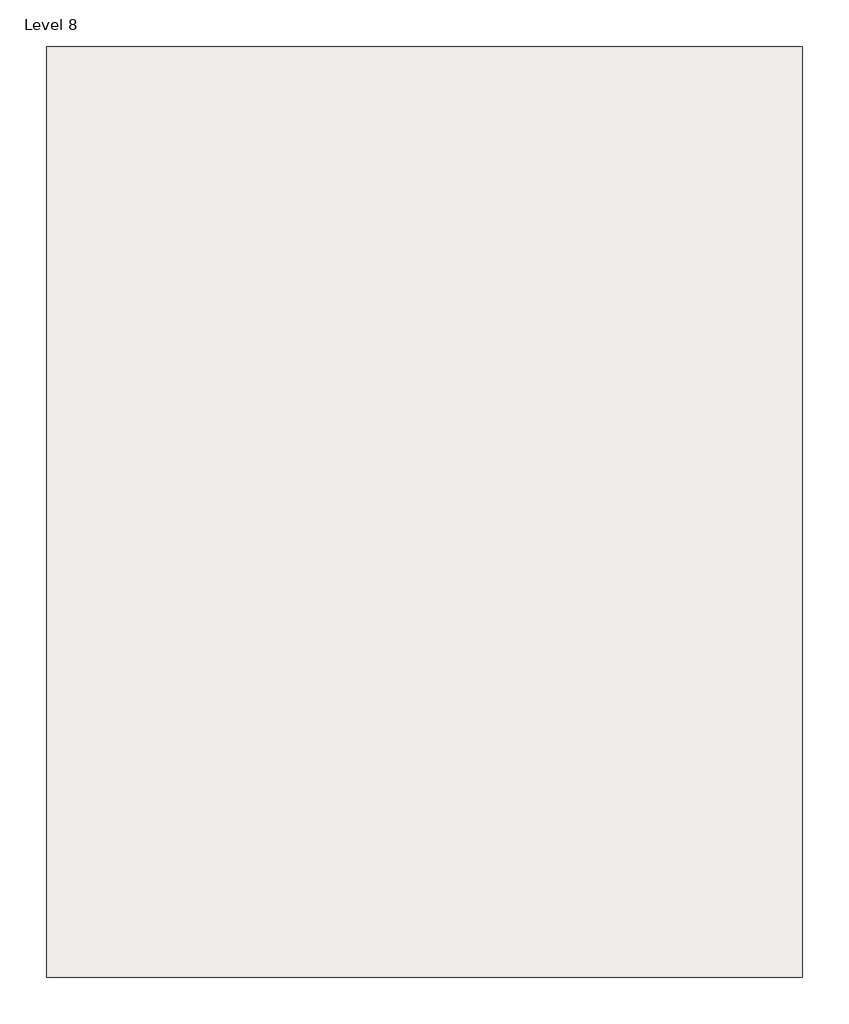
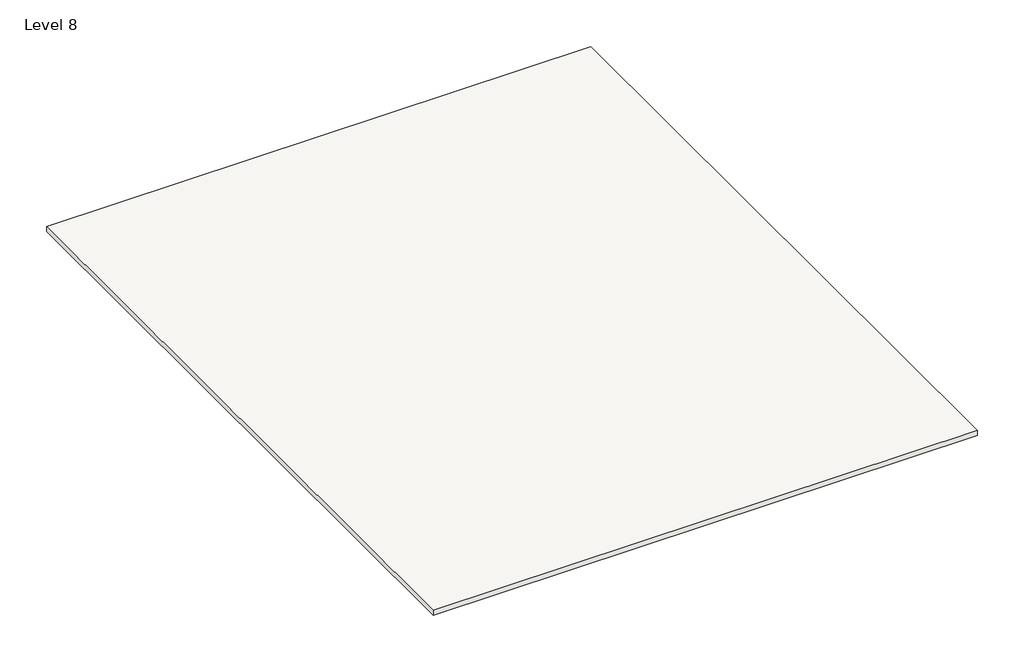
# One storey: 1 roof.
"""IFC4 building model written with IfcOpenShell, lengths in millimetres."""

from ifc_helpers import new_model, si_unit, frame, origin, place, context, project, spatial, polyline, outline, extrude, element, save

model = new_model("IFC4")

# Units and contexts
model_context = context("Model", 3, world=origin())
ifc_project = project(units=[si_unit("LENGTHUNIT", "METRE", prefix="MILLI")], contexts=[model_context])

# Site, building, storey
site = spatial("IfcSite", under=ifc_project)
building = spatial("IfcBuilding", under=site)
storey = spatial("IfcBuildingStorey", under=building, Name="Level 8", Elevation=12649.2)

# Roof
placement = place(None, origin())
element("IfcRoof", 1, ObjectType="6", at=placement, inside=storey, context=model_context, shape_type="SweptSolid", body=[
    extrude(outline(polyline([(74.1689082, 14608.7600271), (15923.7689082, 14608.7600271), (15923.7689082, -4898.4399729), (74.1689082, -4898.4399729), (74.1689082, 14608.7600271)])), frame((0.0, 0.0, 12649.2), z_axis=(0.0, 0.0, 1.0), x_axis=(1.0, 0.0, 0.0)), (0.0, 0.0, 1.0), 152.4),
])

save(model, "model.ifc")

# Revit data of these elements
# Type "6"
#   Assembly Code = "B1020"
#   Layers, outside or top first: 0' - 6" no material (function 1)
# Element 1 (IfcRoof, "6")
#   built-in parameter 1001705 = 42 (stored number, unit not read)
#   built-in parameter 1001710 = 33615
#   Phase Created = New Construction
#   Materials on its faces: "Default Roof"
# Materials
#   "Default Roof": colour RGB 88 101 114, transparency 0
